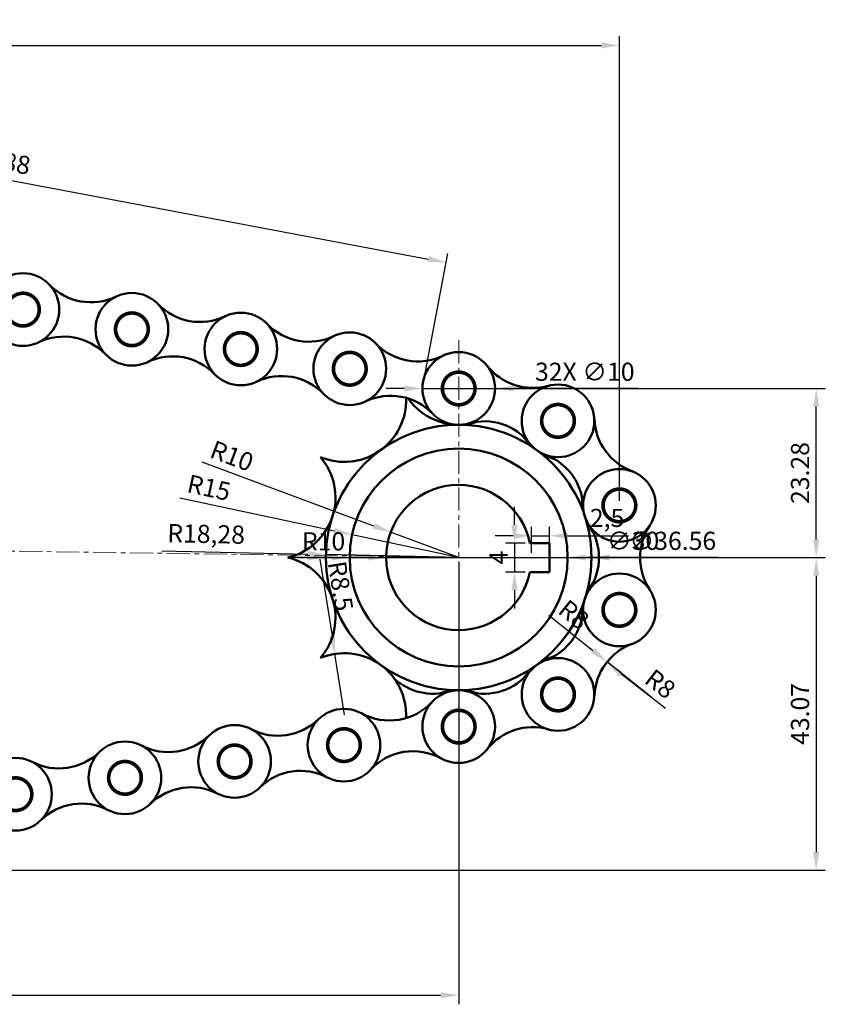
# Model space of a CAD drawing. Units: millimetres. Extents: x 3183 to 3437, y 1388 to 1545.
# Tile 2 of 2: x 3326 to 3437, y 1409 to 1545. Entities that reach past the tile are written whole.
import ezdxf

# ---------------------------------------------------------------- set-up
doc = ezdxf.new("R2010")
doc.units = ezdxf.units.MM
doc.linetypes.add('CENTER', pattern=[50.8, 31.75, -6.35, 6.35, -6.35])
for name, color, linetype, lineweight in [('M-CNTR', 1, 'CENTER', 18), ('M-DIMS', 2, 'Continuous', 25), ('M-OUTL', 7, 'Continuous', 50)]:
    doc.layers.add(name, color=color, linetype=linetype, lineweight=lineweight)
doc.styles.get("Standard").update_dxf_attribs({"font": 'arial.ttf'})
doc.dimstyles.new('ISO-25', dxfattribs={"dimtxt": 2.5, "dimasz": 2.5, "dimexe": 1.25, "dimexo": 0.625, "dimtad": 1, "dimtxsty": 'Standard', "dimcen": 2.5, "dimadec": 0, "dimazin": 0, "dimtfac": 1, "dimtmove": 0, "dimatfit": 3, "dimfxl": 1, "dimarcsym": 0})

# ---------------------------------------------------------------- blocks, each defined once
blk = doc.blocks.new('*D8')
at = {"layer": 'Defpoints', "color": 0, "transparency": 16777216}
for p in [(3398.58, 1473.66), (3396.08, 1470.66), (3398.58, 1470.66)]:
    blk.add_point(p, dxfattribs=at)
at = {"layer": 'M-DIMS', "color": 0, "lineweight": -2, "transparency": 16777216}
for p, q in [((3396.08, 1471.29), (3396.08, 1474.91)), ((3398.58, 1471.29), (3398.58, 1474.91)), ((3393.58, 1473.66), (3391.08, 1473.66)), ((3396.08, 1473.66), (3398.58, 1473.66)), ((3401.08, 1473.66), (3409.44, 1473.66))]:
    blk.add_line(p, q, dxfattribs=at)
at = {"layer": 'M-DIMS', "color": 0, "transparency": 16777216}
for points in [[(3393.58, 1474.08), (3393.58, 1473.24), (3396.08, 1473.66)], [(3401.08, 1474.08), (3401.08, 1473.24), (3398.58, 1473.66)]]:
    blk.add_solid(points, dxfattribs=at)
at = {"layer": 'M-DIMS', "color": 0, "transparency": 16777216, "insert": (3406.51, 1475.79), "char_height": 2.5, "attachment_point": 5}
blk.add_mtext('2,5', dxfattribs=at)
blk = doc.blocks.new('*D9')
at = {"layer": 'Defpoints', "color": 0, "transparency": 16777216}
for p in [(3395.88, 1472.66), (3393.76, 1468.66), (3395.88, 1468.66)]:
    blk.add_point(p, dxfattribs=at)
at = {"layer": 'M-DIMS', "color": 0, "lineweight": -2, "transparency": 16777216}
for p, q in [((3393.76, 1475.16), (3393.76, 1477.66)), ((3395.25, 1472.66), (3392.51, 1472.66)), ((3393.76, 1472.66), (3393.76, 1468.66)), ((3395.25, 1468.66), (3392.51, 1468.66)), ((3393.76, 1466.16), (3393.76, 1463.66))]:
    blk.add_line(p, q, dxfattribs=at)
at = {"layer": 'M-DIMS', "color": 0, "transparency": 16777216}
for points in [[(3393.34, 1475.16), (3394.18, 1475.16), (3393.76, 1472.66)], [(3393.34, 1466.16), (3394.18, 1466.16), (3393.76, 1468.66)]]:
    blk.add_solid(points, dxfattribs=at)
at = {"layer": 'M-DIMS', "color": 0, "transparency": 16777216, "insert": (3391.88, 1470.66), "char_height": 2.5, "attachment_point": 5, "rotation": 90}
blk.add_mtext('4', dxfattribs=at)
blk = doc.blocks.new('*D11')
at = {"layer": 'Defpoints', "color": 0, "transparency": 16777216}
for p in [(3406.44, 1456.2), (3412.75, 1451.29)]:
    blk.add_point(p, dxfattribs=at)
at = {"layer": 'M-DIMS', "color": 0, "lineweight": -2, "transparency": 16777216}
blk.add_line((3414.56, 1449.88), (3408.41, 1454.66), dxfattribs=at)
at = {"layer": 'M-DIMS', "color": 0, "transparency": 16777216}
blk.add_solid([(3408.67, 1454.99), (3408.15, 1454.33), (3406.44, 1456.2)], dxfattribs=at)
at = {"layer": 'M-DIMS', "color": 0, "transparency": 16777216, "insert": (3413.64, 1453.01), "char_height": 2.5, "attachment_point": 5, "rotation": 322.134}
blk.add_mtext('R8', dxfattribs=at)
blk = doc.blocks.new('*D12')
at = {"layer": 'Defpoints', "color": 0, "transparency": 16777216}
for p in [(3376.71, 1474.15), (3386.08, 1470.66)]:
    blk.add_point(p, dxfattribs=at)
at = {"layer": 'M-DIMS', "color": 0, "lineweight": -2, "transparency": 16777216}
for p, q in [((3350.7, 1483.83), (3374.36, 1475.02)), ((3386.08, 1470.66), (3376.71, 1474.15))]:
    blk.add_line(p, q, dxfattribs=at)
at = {"layer": 'M-DIMS', "color": 0, "transparency": 16777216}
blk.add_solid([(3374.51, 1475.41), (3374.22, 1474.63), (3376.71, 1474.15)], dxfattribs=at)
at = {"layer": 'M-DIMS', "color": 0, "transparency": 16777216, "insert": (3354.74, 1484.35), "char_height": 2.5, "attachment_point": 5, "rotation": 339.5937}
blk.add_mtext('R10', dxfattribs=at)
blk = doc.blocks.new('*D13')
at = {"layer": 'Defpoints', "color": 0, "transparency": 16777216}
for p in [(3371.41, 1473.8), (3386.08, 1470.66)]:
    blk.add_point(p, dxfattribs=at)
at = {"layer": 'M-DIMS', "color": 0, "lineweight": -2, "transparency": 16777216}
for p, q in [((3347.69, 1478.87), (3368.97, 1474.32)), ((3386.08, 1470.66), (3371.41, 1473.8))]:
    blk.add_line(p, q, dxfattribs=at)
at = {"layer": 'M-DIMS', "color": 0, "transparency": 16777216}
blk.add_solid([(3369.05, 1474.73), (3368.88, 1473.92), (3371.41, 1473.8)], dxfattribs=at)
at = {"layer": 'M-DIMS', "color": 0, "transparency": 16777216, "insert": (3351.63, 1479.97), "char_height": 2.5, "attachment_point": 5, "rotation": 347.929}
blk.add_mtext('R15', dxfattribs=at)
blk = doc.blocks.new('*D14')
at = {"layer": 'Defpoints', "color": 0, "transparency": 16777216}
for p in [(3367.8, 1471.08), (3386.08, 1470.66)]:
    blk.add_point(p, dxfattribs=at)
at = {"layer": 'M-DIMS', "color": 0, "lineweight": -2, "transparency": 16777216}
for p, q in [((3345.21, 1471.6), (3365.31, 1471.14)), ((3386.08, 1470.66), (3367.8, 1471.08))]:
    blk.add_line(p, q, dxfattribs=at)
at = {"layer": 'M-DIMS', "color": 0, "transparency": 16777216}
blk.add_solid([(3365.31, 1471.56), (3365.3, 1470.72), (3367.8, 1471.08)], dxfattribs=at)
at = {"layer": 'M-DIMS', "color": 0, "transparency": 16777216, "insert": (3351.3, 1473.59), "char_height": 2.5, "attachment_point": 5, "rotation": 358.6875}
blk.add_mtext('R18,28', dxfattribs=at)
blk = doc.blocks.new('*D15')
at = {"layer": 'Defpoints', "color": 0, "transparency": 16777216}
for p in [(3255.4, 1517.6), (3384.35, 1511.3), (3381.08, 1493.94)]:
    blk.add_point(p, dxfattribs=at)
at = {"layer": 'M-DIMS', "color": 0, "lineweight": -2, "transparency": 16777216}
for p, q in [((3255.52, 1518.21), (3258.9, 1536.18)), ((3261.13, 1534.49), (3381.89, 1511.76)), ((3381.2, 1494.56), (3384.58, 1512.53))]:
    blk.add_line(p, q, dxfattribs=at)
at = {"layer": 'M-DIMS', "color": 0, "transparency": 16777216}
for points in [[(3261.2, 1534.9), (3261.05, 1534.08), (3258.67, 1534.95)], [(3381.97, 1512.17), (3381.81, 1511.35), (3384.35, 1511.3)]]:
    blk.add_solid(points, dxfattribs=at)
at = {"layer": 'M-DIMS', "color": 0, "transparency": 16777216, "insert": (3321.9, 1525.22), "char_height": 2.5, "attachment_point": 5, "rotation": 349.3415}
blk.add_mtext('127,88', dxfattribs=at)
blk = doc.blocks.new('CHAIN-ROLLER')
at = {"const_width": 0.5}
blk.add_lwpolyline([(3252.61, 1517.82, 1), (3248.13, 1517.37, 1)], format="xyb", close=True, dxfattribs=at)
blk.add_circle((3250.37, 1517.59), 5)
blk = doc.blocks.new('CHAIN-ROLLER-B')
at = {"const_width": 0.5}
blk.add_lwpolyline([(3262.52, 1429.27, -1), (3267, 1428.86, -1)], format="xyb", close=True, dxfattribs=at)
blk.add_circle((3264.76, 1429.06), 5)
blk = doc.blocks.new('*D22')
at = {"layer": 'Defpoints', "color": 0, "transparency": 16777216}
for p in [(3250.4, 1472.6), (3386.08, 1470.66), (3386.08, 1410.4)]:
    blk.add_point(p, dxfattribs=at)
at = {"layer": 'M-DIMS', "color": 0, "lineweight": -2, "transparency": 16777216}
for p, q in [((3250.4, 1471.97), (3250.4, 1409.15)), ((3386.08, 1470.04), (3386.08, 1409.15)), ((3252.9, 1410.4), (3383.58, 1410.4))]:
    blk.add_line(p, q, dxfattribs=at)
at = {"layer": 'M-DIMS', "color": 0, "transparency": 16777216}
for points in [[(3252.9, 1410.81), (3252.9, 1409.98), (3250.4, 1410.4)], [(3383.58, 1410.81), (3383.58, 1409.98), (3386.08, 1410.4)]]:
    blk.add_solid(points, dxfattribs=at)
at = {"layer": 'M-DIMS', "color": 0, "transparency": 16777216, "insert": (3318.24, 1412.3), "char_height": 2.5, "attachment_point": 5}
blk.add_mtext('135.68', dxfattribs=at)
blk = doc.blocks.new('*D23')
at = {"layer": 'Defpoints', "color": 0, "transparency": 16777216}
for p in [(3386.08, 1470.66), (3250.4, 1427.6), (3435.3, 1427.6)]:
    blk.add_point(p, dxfattribs=at)
at = {"layer": 'M-DIMS', "color": 0, "lineweight": -2, "transparency": 16777216}
for p, q in [((3386.7, 1470.66), (3436.55, 1470.66)), ((3435.3, 1468.16), (3435.3, 1430.1)), ((3251.03, 1427.6), (3436.55, 1427.6))]:
    blk.add_line(p, q, dxfattribs=at)
at = {"layer": 'M-DIMS', "color": 0, "transparency": 16777216}
for points in [[(3434.89, 1468.16), (3435.72, 1468.16), (3435.3, 1470.66)], [(3434.89, 1430.1), (3435.72, 1430.1), (3435.3, 1427.6)]]:
    blk.add_solid(points, dxfattribs=at)
at = {"layer": 'M-DIMS', "color": 0, "transparency": 16777216, "insert": (3433.4, 1449.13), "char_height": 2.5, "attachment_point": 5, "rotation": 90}
blk.add_mtext('43.07', dxfattribs=at)
blk = doc.blocks.new('*D24')
at = {"layer": 'Defpoints', "color": 0, "transparency": 16777216}
for p in [(3408.21, 1541.18), (3206.09, 1480.41), (3408.21, 1477.84)]:
    blk.add_point(p, dxfattribs=at)
at = {"layer": 'M-DIMS', "color": 0, "lineweight": -2, "transparency": 16777216}
for p, q in [((3206.09, 1481.04), (3206.09, 1542.43)), ((3408.21, 1478.47), (3408.21, 1542.43)), ((3208.59, 1541.18), (3405.71, 1541.18))]:
    blk.add_line(p, q, dxfattribs=at)
at = {"layer": 'M-DIMS', "color": 0, "transparency": 16777216}
for points in [[(3208.59, 1541.59), (3208.59, 1540.76), (3206.09, 1541.18)], [(3405.71, 1541.59), (3405.71, 1540.76), (3408.21, 1541.18)]]:
    blk.add_solid(points, dxfattribs=at)
at = {"layer": 'M-DIMS', "color": 0, "transparency": 16777216, "insert": (3307.15, 1543.08), "char_height": 2.5, "attachment_point": 5}
blk.add_mtext('202.1', dxfattribs=at)
blk = doc.blocks.new('*D26')
at = {"layer": 'Defpoints', "color": 0, "transparency": 16777216}
for p in [(3386.08, 1493.94), (3435.3, 1493.94), (3386.08, 1470.66)]:
    blk.add_point(p, dxfattribs=at)
at = {"layer": 'M-DIMS', "color": 0, "lineweight": -2, "transparency": 16777216}
for p, q in [((3386.7, 1493.94), (3436.55, 1493.94)), ((3435.3, 1473.16), (3435.3, 1491.44)), ((3386.7, 1470.66), (3436.55, 1470.66))]:
    blk.add_line(p, q, dxfattribs=at)
at = {"layer": 'M-DIMS', "color": 0, "transparency": 16777216}
for points in [[(3434.89, 1491.44), (3435.72, 1491.44), (3435.3, 1493.94)], [(3434.89, 1473.16), (3435.72, 1473.16), (3435.3, 1470.66)]]:
    blk.add_solid(points, dxfattribs=at)
at = {"layer": 'M-DIMS', "color": 0, "transparency": 16777216, "insert": (3433.4, 1482.3), "char_height": 2.5, "attachment_point": 5, "rotation": 90}
blk.add_mtext('23.28', dxfattribs=at)
blk = doc.blocks.new('*D35')
at = {"layer": 'Defpoints', "color": 0, "transparency": 16777216}
for p in [(3367.8, 1470.66), (3404.36, 1470.66)]:
    blk.add_point(p, dxfattribs=at)
at = {"layer": 'M-DIMS', "color": 0, "lineweight": -2, "transparency": 16777216}
for p, q in [((3365.3, 1470.66), (3362.8, 1470.66)), ((3367.8, 1470.66), (3404.36, 1470.66)), ((3421.76, 1470.66), (3406.86, 1470.66))]:
    blk.add_line(p, q, dxfattribs=at)
at = {"layer": 'M-DIMS', "color": 0, "transparency": 16777216}
for points in [[(3365.3, 1471.08), (3365.3, 1470.25), (3367.8, 1470.66)], [(3406.86, 1471.08), (3406.86, 1470.25), (3404.36, 1470.66)]]:
    blk.add_solid(points, dxfattribs=at)
at = {"layer": 'M-DIMS', "color": 0, "transparency": 16777216, "insert": (3415.56, 1472.64), "char_height": 2.5, "attachment_point": 5, "rotation": 0.0013}
blk.add_mtext('∅36.56', dxfattribs=at)
blk = doc.blocks.new('*D36')
at = {"layer": 'Defpoints', "color": 0, "transparency": 16777216}
for p in [(3371.08, 1470.66), (3401.08, 1470.66)]:
    blk.add_point(p, dxfattribs=at)
at = {"layer": 'M-DIMS', "color": 0, "lineweight": -2, "transparency": 16777216}
for p, q in [((3368.58, 1470.66), (3366.08, 1470.66)), ((3371.08, 1470.66), (3401.08, 1470.66)), ((3413.85, 1470.66), (3403.58, 1470.66))]:
    blk.add_line(p, q, dxfattribs=at)
at = {"layer": 'M-DIMS', "color": 0, "transparency": 16777216}
for points in [[(3368.58, 1471.08), (3368.58, 1470.25), (3371.08, 1470.66)], [(3403.58, 1471.08), (3403.58, 1470.25), (3401.08, 1470.66)]]:
    blk.add_solid(points, dxfattribs=at)
at = {"layer": 'M-DIMS', "color": 0, "transparency": 16777216, "insert": (3410.08, 1472.64), "char_height": 2.5, "attachment_point": 5, "rotation": 0.0016}
blk.add_mtext('∅30', dxfattribs=at)
blk = doc.blocks.new('*D37')
at = {"layer": 'Defpoints', "color": 0, "transparency": 16777216}
for p in [(3376.08, 1470.66), (3386.08, 1470.66)]:
    blk.add_point(p, dxfattribs=at)
at = {"layer": 'M-DIMS', "color": 0, "lineweight": -2, "transparency": 16777216}
for p, q in [((3363.86, 1470.66), (3373.58, 1470.66)), ((3386.08, 1470.66), (3376.08, 1470.66))]:
    blk.add_line(p, q, dxfattribs=at)
at = {"layer": 'M-DIMS', "color": 0, "transparency": 16777216}
blk.add_solid([(3373.58, 1471.08), (3373.58, 1470.25), (3376.08, 1470.66)], dxfattribs=at)
at = {"layer": 'M-DIMS', "color": 0, "transparency": 16777216, "insert": (3367.47, 1472.57), "char_height": 2.5, "attachment_point": 5, "rotation": 359.9977}
blk.add_mtext('R10', dxfattribs=at)
blk = doc.blocks.new('*D38')
at = {"layer": 'Defpoints', "color": 0, "transparency": 16777216}
for p in [(3369.03, 1457.4), (3370.34, 1449)]:
    blk.add_point(p, dxfattribs=at)
at = {"layer": 'M-DIMS', "color": 0, "lineweight": -2, "transparency": 16777216}
for p, q in [((3366.98, 1470.45), (3368.64, 1459.87)), ((3370.34, 1449), (3369.03, 1457.4))]:
    blk.add_line(p, q, dxfattribs=at)
at = {"layer": 'M-DIMS', "color": 0, "transparency": 16777216}
blk.add_solid([(3369.05, 1459.93), (3368.23, 1459.8), (3369.03, 1457.4)], dxfattribs=at)
at = {"layer": 'M-DIMS', "color": 0, "transparency": 16777216, "insert": (3369.5, 1466.69), "char_height": 2.5, "attachment_point": 5, "rotation": 278.8928}
blk.add_mtext('R8.5', dxfattribs=at)
blk = doc.blocks.new('*D39')
at = {"layer": 'Defpoints', "color": 0, "transparency": 16777216}
for p in [(3406.51, 1456.29), (3412.75, 1451.29)]:
    blk.add_point(p, dxfattribs=at)
at = {"layer": 'M-DIMS', "color": 0, "lineweight": -2, "transparency": 16777216}
for p, q in [((3398.49, 1462.73), (3404.56, 1457.86)), ((3412.75, 1451.29), (3406.51, 1456.29))]:
    blk.add_line(p, q, dxfattribs=at)
at = {"layer": 'M-DIMS', "color": 0, "transparency": 16777216}
blk.add_solid([(3404.82, 1458.18), (3404.3, 1457.53), (3406.51, 1456.29)], dxfattribs=at)
at = {"layer": 'M-DIMS', "color": 0, "transparency": 16777216, "insert": (3401.74, 1462.56), "char_height": 2.5, "attachment_point": 5, "rotation": 321.2529}
blk.add_mtext('R8', dxfattribs=at)
blk = doc.blocks.new('*D40')
at = {"layer": 'Defpoints', "color": 0, "transparency": 16777216}
for p in [(3381.08, 1493.94), (3391.08, 1493.94)]:
    blk.add_point(p, dxfattribs=at)
at = {"layer": 'M-DIMS', "color": 0, "lineweight": -2, "transparency": 16777216}
for p, q in [((3378.58, 1493.94), (3376.08, 1493.94)), ((3381.08, 1493.94), (3391.08, 1493.94)), ((3410.8, 1493.95), (3393.58, 1493.94))]:
    blk.add_line(p, q, dxfattribs=at)
at = {"layer": 'M-DIMS', "color": 0, "transparency": 16777216}
for points in [[(3378.58, 1494.36), (3378.58, 1493.53), (3381.08, 1493.94)], [(3393.58, 1494.36), (3393.58, 1493.53), (3391.08, 1493.94)]]:
    blk.add_solid(points, dxfattribs=at)
at = {"layer": 'M-DIMS', "color": 0, "transparency": 16777216, "insert": (3403.44, 1495.92), "char_height": 2.5, "attachment_point": 5, "rotation": 0.0047}
blk.add_mtext('32X ∅10', dxfattribs=at)

msp = doc.modelspace()

# ---------------------------------------------------------------- linework, layer by layer
at = {"layer": 'M-CNTR', "ltscale": 0.1}
msp.add_line((3386.08, 1500.6139), (3386.08, 1439.2736), dxfattribs=at)
msp.add_lwpolyline([(3203.6712, 1473.2614), (3386.08, 1470.6636), (3423.1034, 1470.6522)], dxfattribs=at)
at = {"layer": 'M-OUTL'}
for p, q in [((3398.58, 1472.6636), (3395.8779, 1472.6636)), ((3398.58, 1470.6636), (3398.58, 1472.6636)), ((3398.58, 1470.6636), (3398.58, 1468.6636)), ((3398.58, 1468.6636), (3395.8779, 1468.6636))]:
    msp.add_line(p, q, dxfattribs=at)
at = {"layer": 'M-OUTL', "const_width": 0.5}
msp.add_lwpolyline([(3383.83, 1493.9436, 1), (3388.33, 1493.9436, 1)], format="xyb", close=True, dxfattribs=at)
at = {"layer": 'M-OUTL'}
for centre, radius in [((3386.08, 1493.9436), 5), ((3386.08, 1493.9436), 5), ((3386.08, 1470.6636), 18.28), ((3386.08, 1470.6636), 15)]:
    msp.add_circle(centre, radius, dxfattribs=at)
for centre, radius, start, end in [((3335.4557, 1513.809), 8, 223.845854, 295.635223), ((3350.4557, 1511.094), 8, 223.845854, 295.635223), ((3365.4557, 1508.379), 8, 223.845854, 295.635223), ((3331.7043, 1493.0832), 8, 43.845854, 115.635223), ((3380.4557, 1505.664), 8, 223.845854, 295.635223), ((3346.7043, 1490.3682), 8, 43.845854, 115.635223), ((3396.2679, 1502.0187), 8, 218.400923, 285.599077), ((3361.7043, 1487.6532), 8, 43.845854, 115.635223), ((3376.7043, 1484.9382), 8, 43.845854, 115.635223), ((3370.3391, 1492.3291), 8.5, 247.198393, 2.162508), ((3386.08, 1497.4436), 8.5, 215.026636, 288.488301), ((3386.08, 1497.4436), 8.5, 251.511699, 288.488301), ((3389.5757, 1481.4224), 8, 38.400923, 105.599077), ((3412.7522, 1490.0421), 8, 182.400923, 249.599077), ((3370.3391, 1492.3291), 8.5, 259.603963, 324.488301), ((3401.8209, 1492.3291), 8.5, 215.511699, 252.488301), ((3395.232, 1477.3129), 8, 12.258582, 69.599077), ((3360.6107, 1478.9391), 8.5, 283.198393, 40.801607), ((3386.08, 1470.6636), 10, 11.536959, 348.463041), ((3411.5493, 1478.9391), 8.5, 179.511699, 216.488301), ((3395.232, 1477.3129), 8, 357.772121, 359.12383), ((3397.3925, 1470.6636), 8, 326.400923, 33.599077), ((3419.0487, 1470.6636), 8, 146.400923, 213.599077), ((3360.6107, 1462.3881), 8.5, 319.198393, 76.801607), ((3411.5493, 1462.3881), 8.5, 143.511699, 180.488301), ((3395.232, 1464.0143), 8, 290.400923, 347.741418), ((3412.7522, 1451.2851), 8, 110.400923, 177.599077), ((3370.3391, 1448.9981), 8.5, 357.018663, 112.801607), ((3401.8209, 1448.9981), 8.5, 107.511699, 144.488301), ((3389.5757, 1459.9048), 8, 254.400923, 321.599077), ((3382.5842, 1459.9048), 8, 228.258582, 285.599077), ((3386.08, 1443.8836), 8.5, 71.511699, 108.488301), ((3376.5493, 1456.2248), 8, 241.183338, 317.149357), ((3361.1888, 1454.1239), 8, 242.603084, 314.392454), ((3396.2679, 1439.3085), 8, 74.400923, 141.599077), ((3346.1124, 1451.8714), 8, 242.603084, 314.392454), ((3331.0361, 1449.6188), 8, 242.603084, 314.392454), ((3379.8139, 1435.9934), 8, 61.183338, 137.149357), ((3364.3012, 1433.2927), 8, 62.603084, 134.392454), ((3349.2249, 1431.0401), 8, 62.603084, 134.392454), ((3334.1485, 1428.7875), 8, 62.603084, 134.392454)]:
    msp.add_arc(centre, radius, start, end, dxfattribs=at)

# ---------------------------------------------------------------- block references
for name, p, rotation in [('CHAIN-ROLLER', (6711.5203, 2690.8868), 174.2800065540113), ('CHAIN-ROLLER', (6726.5203, 2688.1718), 174.2800065540054), ('CHAIN-ROLLER', (6741.5203, 2685.4568), 174.2800065540229), ('CHAIN-ROLLER', (6756.5203, 2682.7418), 174.2800065540223), ('CHAIN-ROLLER', (4959.2734, -1740.9805), 90.7413947143664), ('CHAIN-ROLLER', (4967.7303, -1752.6205), 90.74139471438066), ('CHAIN-ROLLER', (4967.7303, -1767.0083), 90.74139471437879), ('CHAIN-ROLLER', (4959.2734, -1778.6483), 90.74139471436543), ('CHAIN-ROLLER-B', (212.0423, -173.2246), 3.407903634777628), ('CHAIN-ROLLER-B', (196.2455, -175.7736), 3.407903634794749), ('CHAIN-ROLLER-B', (166.0927, -180.2788), 3.407903634793037), ('CHAIN-ROLLER-B', (151.0164, -182.5314), 3.407903634794214)]:
    msp.add_blockref(name, p, dxfattribs=dict(at, rotation=rotation))
at = {"layer": 'M-OUTL', "extrusion": (0, 0, -1), "zscale": -1, "rotation": 180.1085086200507}
msp.add_blockref('CHAIN-ROLLER-B', (-93.1825, 2877.83), dxfattribs=at)

# ---------------------------------------------------------------- dimensions: what is measured, and where the dimension line sits
at = {"layer": 'M-DIMS'}
for base, p1, p2, override, picture, middle in [((3408.2054, 1541.1774), (3206.0883, 1480.41), (3408.2054, 1477.841), {"dimdec": 1, "dimlfac": 1, "dimrnd": 0, "dimzin": 0, "dimdsep": 46, "dimlunit": 2}, '*D24', (3307.1468, 1543.0788)), ((3398.58, 1473.6601), (3396.08, 1470.6636), (3398.58, 1470.6636), {"dimclrd": 0, "dimclre": 0, "dimclrt": 0}, '*D8', (3406.5114, 1475.7875)), ((3386.08, 1410.3958), (3250.4046, 1472.5958), (3386.08, 1470.6636), {"dimdec": 2, "dimlfac": 1, "dimrnd": 0, "dimzin": 0, "dimdsep": 46, "dimlunit": 2}, '*D22', (3318.2423, 1412.2981))]:
    dim = msp.add_linear_dim(base=base, p1=p1, p2=p2, dimstyle='ISO-25', override=override, dxfattribs=at)
    dim.commit()
    dim.dimension.update_dxf_attribs({"geometry": picture, "text_midpoint": middle})
dim = msp.add_aligned_dim(p1=(3255.4046, 1517.5958), p2=(3381.08, 1493.9436), distance=17.6603, dimstyle='ISO-25', override={"dimclrd": 0, "dimclre": 0, "dimclrt": 0}, dxfattribs=at)
dim.commit()
dim.dimension.update_dxf_attribs({"geometry": '*D15', "text_midpoint": (3321.9021, 1525.216)})
dim = msp.add_diameter_dim_2p(p1=(3381.08, 1493.9432), p2=(3391.08, 1493.944), text='32X <>', dimstyle='ISO-25', override={"dimdec": 0, "dimlfac": 1, "dimrnd": 0, "dimzin": 0, "dimdsep": 46, "dimlunit": 2}, dxfattribs=at)
dim.commit()
dim.dimension.update_dxf_attribs({"geometry": '*D40', "text_midpoint": (3403.441, 1493.945), "dimtype": 163})
for base, p1, p2, override, picture, middle in [((3435.3034, 1493.9436), (3386.08, 1470.6636), (3386.08, 1493.9436), {"dimdec": 2, "dimlfac": 1, "dimrnd": 0, "dimzin": 0, "dimdsep": 46, "dimlunit": 2}, '*D26', (3433.4011, 1482.3036)), ((3393.7586, 1468.6636), (3395.8779, 1472.6636), (3395.8779, 1468.6636), {"dimclrd": 0, "dimclre": 0, "dimclrt": 0}, '*D9', (3391.8836, 1470.6636)), ((3435.3034, 1427.5958), (3386.08, 1470.6636), (3250.4046, 1427.5958), {"dimdec": 2, "dimlfac": 1, "dimrnd": 0, "dimzin": 0, "dimdsep": 46, "dimlunit": 2}, '*D23', (3433.4011, 1449.1297))]:
    dim = msp.add_linear_dim(base=base, p1=p1, p2=p2, angle=90, dimstyle='ISO-25', override=override, dxfattribs=at)
    dim.commit()
    dim.dimension.update_dxf_attribs({"geometry": picture, "text_midpoint": middle})
for center, mpoint, picture, middle in [((3386.08, 1470.6636), (3376.7076, 1474.1503), '*D12', (3354.0763, 1482.5697)), ((3386.08, 1470.6636), (3371.4117, 1473.8004), '*D13', (3351.2352, 1478.1152)), ((3386.08, 1470.6636), (3367.8048, 1471.0823), '*D14', (3351.254, 1471.4615)), ((3412.7522, 1451.2851), (3406.4366, 1456.1956), '*D11', (3412.4706, 1451.5041))]:
    dim = msp.add_radius_dim(center=center, mpoint=mpoint, dimstyle='ISO-25', override={"dimclrd": 0, "dimclre": 0, "dimclrt": 0}, dxfattribs=at)
    dim.commit()
    dim.dimension.update_dxf_attribs({"geometry": picture, "text_midpoint": middle, "dimtype": 164})
dim = msp.add_diameter_dim_2p(p1=(3367.8, 1470.6632), p2=(3404.36, 1470.664), dimstyle='ISO-25', override={"dimdec": 2, "dimlfac": 1, "dimrnd": 0, "dimzin": 0, "dimdsep": 46, "dimlunit": 2}, dxfattribs=at)
dim.commit()
dim.dimension.update_dxf_attribs({"geometry": '*D35', "text_midpoint": (3415.5622, 1470.6643)})
for center, mpoint, override, picture, middle in [((3386.08, 1470.6636), (3376.08, 1470.664), {"dimdec": 0, "dimlfac": 1, "dimrnd": 0, "dimzin": 0, "dimdsep": 46, "dimlunit": 2}, '*D37', (3367.4725, 1472.5658)), ((3370.3391, 1448.9981), (3369.0251, 1457.3959), {"dimdec": 1, "dimlfac": 1, "dimrnd": 0, "dimzin": 0, "dimdsep": 46, "dimlunit": 2}, '*D38', (3369.496, 1466.6868)), ((3412.7522, 1451.2851), (3406.5129, 1456.2922), {"dimdec": 0, "dimlfac": 1, "dimrnd": 0, "dimzin": 0, "dimdsep": 46, "dimlunit": 2}, '*D39', (3401.7419, 1462.5589))]:
    dim = msp.add_radius_dim(center=center, mpoint=mpoint, dimstyle='ISO-25', override=override, dxfattribs=at)
    dim.commit()
    dim.dimension.update_dxf_attribs({"geometry": picture, "text_midpoint": middle})
dim = msp.add_diameter_dim_2p(p1=(3371.08, 1470.6632), p2=(3401.08, 1470.664), dimstyle='ISO-25', override={"dimdec": 0, "dimlfac": 1, "dimrnd": 0, "dimzin": 0, "dimdsep": 46, "dimlunit": 2}, dxfattribs=at)
dim.commit()
dim.dimension.update_dxf_attribs({"geometry": '*D36', "text_midpoint": (3410.08, 1470.6642), "dimtype": 163})

doc.saveas('drawing.dxf')
